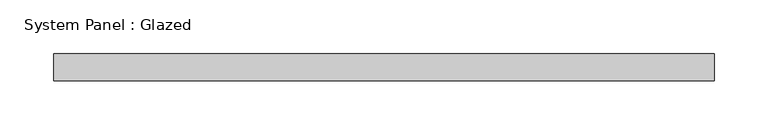
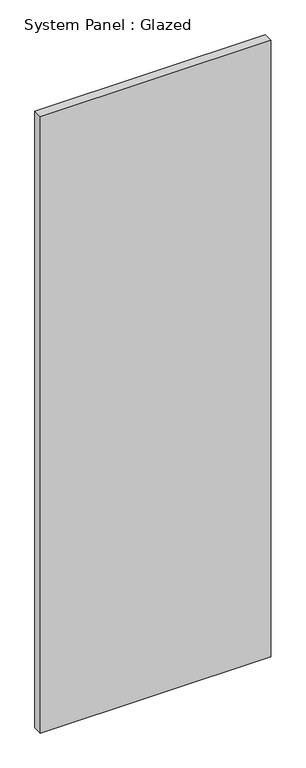
"""IFC4 building model written with IfcOpenShell, lengths in millimetres: plate geometry, System Panel : Glazed."""

from ifc_helpers import new_model, si_unit, origin, origin_with_axes, place, context, project, spatial, polyline, outline, extrude, source, transform, mapped, element, save


def system_panel_glazed_d85bf7d9(model_context):
    return source(origin(), model_context, "Body", "SweptSolid", [
        extrude(outline(polyline([(307.975, 19.05), (-307.975, 19.05), (-307.975, 44.45), (307.975, 44.45), (307.975, 19.05)])), origin_with_axes(), (0.0, 0.0, 1.0), 1741.0529055),
    ])


if __name__ == "__main__":
    model = new_model("IFC4")
    model_context = context("Model", 3, world=origin())
    ifc_project = project(units=[si_unit("LENGTHUNIT", "METRE", prefix="MILLI")], contexts=[model_context])
    site = spatial("IfcSite", under=ifc_project)
    building = spatial("IfcBuilding", under=site)
    placement = place(None, origin())
    system_panel_glazed_shape = system_panel_glazed_d85bf7d9(model_context)
    element("IfcPlate", 1, ObjectType="System Panel : Glazed", at=placement, inside=building, context=model_context, shape_type="MappedRepresentation", body=[
        mapped(system_panel_glazed_shape, transform((0.0, 0.0, 0.0), x_axis=(1.0, 0.0, 0.0), y_axis=(0.0, 1.0, 0.0), z_axis=(0.0, 0.0, 1.0))),
    ])
    save(model, "model.ifc")

# Revit data of these elements
# Type "System Panel : Glazed"
#   Construction Type Id = "GSP4R"
#   Analytic Construction = "1/8 in Pilkington single glazing"
#   Visual Light Transmittance = 0.9
#   Solar Heat Gain Coefficient = 0.86
#   Heat Transfer Coefficient (U) = 1.18115 BTU/(h·ft²·°F)
#   Define Thermal Properties by = 1
# Element 1 (IfcPlate, "System Panel : Glazed")
#   Materials on its faces: "Glass"
# Materials
#   "Glass": class "Glass", colour RGB 0 128 192, transparency 0.75, Description = "Soda Lime Glass", Cost = 0
